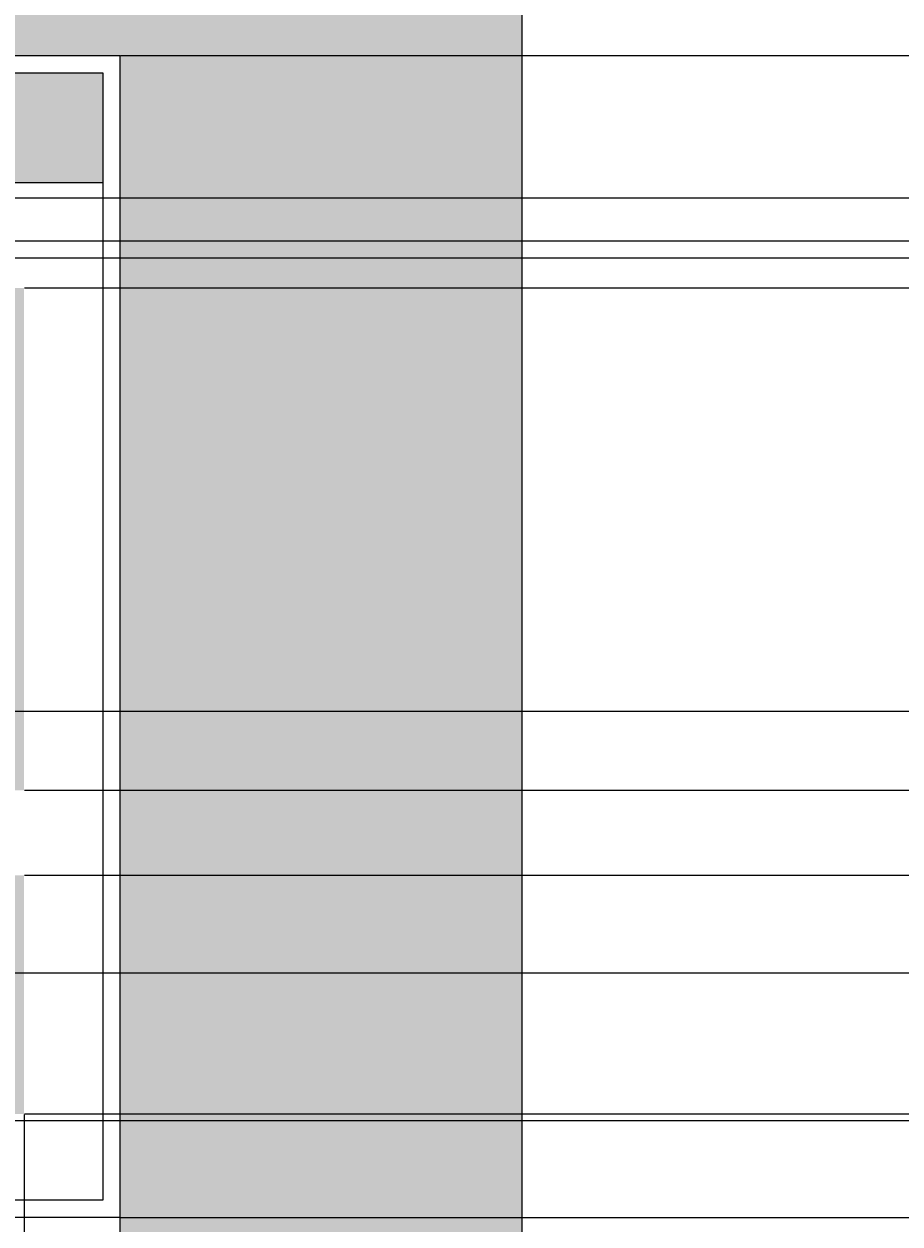
# Model space of a CAD drawing. Units: inches. Extents: x 36 to 594, y 79 to 831.
# Tile 12 of 30: x 390 to 492, y 150 to 290. Entities that reach past the tile are written whole.
import ezdxf

# ---------------------------------------------------------------- set-up
doc = ezdxf.new("R2010")
doc.units = ezdxf.units.IN
doc.header["$MEASUREMENT"] = 0
for name, color, linetype, lineweight in [('A-ANNO-DIMS', 2, 'Continuous', 18), ('A-DOOR', 3, 'Continuous', 18), ('A-ELEV', 7, 'Continuous', 25), ('A-ELEV-PATT', 8, 'Continuous', 13)]:
    doc.layers.add(name, color=color, linetype=linetype, lineweight=lineweight)
doc.styles.get("Standard").update_dxf_attribs({"font": 'arial.ttf'})
doc.dimstyles.get("Standard").update_dxf_attribs({"dimtxt": 0.8125, "dimasz": 0.18, "dimexe": 0.18, "dimexo": 0.0625, "dimgap": 0.09, "dimtad": 0, "dimtih": 1, "dimtoh": 1, "dimdec": 4, "dimzin": 0, "dimdsep": 46, "dimlunit": 4, "dimtxsty": 'Standard', "dimcen": 0.09, "dimadec": 0, "dimazin": 0, "dimtfac": 1, "dimtdec": 4, "dimtofl": 0, "dimtmove": 0, "dimatfit": 3, "dimfxl": 1, "dimtolj": 1, "dimtzin": 0, "dimarcsym": 0})

# ---------------------------------------------------------------- blocks, each defined once
blk = doc.blocks.new('*D30')
at = {"layer": 'A-ANNO-DIMS', "color": 0, "lineweight": -2, "transparency": 16777216}
for p, q in [((401.61, 150.93), (592.85, 150.93)), ((592.67, 150.75), (592.67, 147.08)), ((592.67, 142.39), (592.67, 146.07)), ((401.61, 142.21), (592.85, 142.21))]:
    blk.add_line(p, q, dxfattribs=at)
at = {"layer": 'A-ANNO-DIMS', "color": 0, "transparency": 16777216}
for points in [[(592.64, 150.75), (592.7, 150.75), (592.67, 150.93)], [(592.64, 142.39), (592.7, 142.39), (592.67, 142.21)]]:
    blk.add_solid(points, dxfattribs=at)
at = {"layer": 'Defpoints', "color": 0, "transparency": 16777216}
for p in [(401.55, 150.93), (592.67, 150.93), (401.55, 142.21)]:
    blk.add_point(p, dxfattribs=at)
at = {"layer": 'A-ANNO-DIMS', "color": 0, "transparency": 16777216, "insert": (592.67, 146.57), "char_height": 0.812, "attachment_point": 5}
blk.add_mtext('\\A1;8.722', dxfattribs=at)
blk = doc.blocks.new('*D31')
at = {"layer": 'A-ANNO-DIMS', "color": 0, "lineweight": -2, "transparency": 16777216}
for p, q in [((448.45, 306.21), (592.85, 306.21)), ((592.67, 306.03), (592.67, 229.08)), ((592.67, 151.11), (592.67, 228.07)), ((401.61, 150.93), (592.85, 150.93))]:
    blk.add_line(p, q, dxfattribs=at)
at = {"layer": 'A-ANNO-DIMS', "color": 0, "transparency": 16777216}
for points in [[(592.64, 306.03), (592.7, 306.03), (592.67, 306.21)], [(592.64, 151.11), (592.7, 151.11), (592.67, 150.93)]]:
    blk.add_solid(points, dxfattribs=at)
at = {"layer": 'Defpoints', "color": 0, "transparency": 16777216}
for p in [(448.39, 306.21), (592.67, 306.21), (401.55, 150.93)]:
    blk.add_point(p, dxfattribs=at)
at = {"layer": 'A-ANNO-DIMS', "color": 0, "transparency": 16777216, "insert": (592.67, 228.57), "char_height": 0.812, "attachment_point": 5}
blk.add_mtext('\\A1;155.28', dxfattribs=at)
blk = doc.blocks.new('*D74')
at = {"layer": 'A-ANNO-DIMS', "color": 0, "lineweight": -2, "transparency": 16777216}
for p, q in [((217.09, 179.42), (592.85, 179.42)), ((592.67, 179.24), (592.67, 171.32)), ((592.67, 162.39), (592.67, 170.31)), ((217.09, 162.21), (592.85, 162.21))]:
    blk.add_line(p, q, dxfattribs=at)
at = {"layer": 'A-ANNO-DIMS', "color": 0, "transparency": 16777216}
for points in [[(592.64, 179.24), (592.7, 179.24), (592.67, 179.42)], [(592.64, 162.39), (592.7, 162.39), (592.67, 162.21)]]:
    blk.add_solid(points, dxfattribs=at)
at = {"layer": 'Defpoints', "color": 0, "transparency": 16777216}
for p in [(217.03, 179.42), (592.67, 179.42), (217.03, 162.21)]:
    blk.add_point(p, dxfattribs=at)
at = {"layer": 'A-ANNO-DIMS', "color": 0, "transparency": 16777216, "insert": (592.67, 170.82), "char_height": 0.812, "attachment_point": 5}
blk.add_mtext('\\A1;17.207', dxfattribs=at)
blk = doc.blocks.new('*D75')
at = {"layer": 'A-ANNO-DIMS', "color": 0, "lineweight": -2, "transparency": 16777216}
for p, q in [((215.09, 262.62), (592.85, 262.62)), ((592.67, 262.44), (592.67, 221.53)), ((592.67, 179.6), (592.67, 220.52)), ((217.09, 179.42), (592.85, 179.42))]:
    blk.add_line(p, q, dxfattribs=at)
at = {"layer": 'A-ANNO-DIMS', "color": 0, "transparency": 16777216}
for points in [[(592.64, 262.44), (592.7, 262.44), (592.67, 262.62)], [(592.64, 179.6), (592.7, 179.6), (592.67, 179.42)]]:
    blk.add_solid(points, dxfattribs=at)
at = {"layer": 'Defpoints', "color": 0, "transparency": 16777216}
for p in [(215.03, 262.62), (592.67, 262.62), (217.03, 179.42)]:
    blk.add_point(p, dxfattribs=at)
at = {"layer": 'A-ANNO-DIMS', "color": 0, "transparency": 16777216, "insert": (592.67, 221.02), "char_height": 0.812, "attachment_point": 5}
blk.add_mtext('\\A1;83.2', dxfattribs=at)
blk = doc.blocks.new('*D76')
at = {"layer": 'A-ANNO-DIMS', "color": 0, "lineweight": -2, "transparency": 16777216}
for p, q in [((217.09, 264.62), (592.85, 264.62)), ((592.67, 264.44), (592.67, 264.12)), ((215.09, 262.62), (592.85, 262.62)), ((592.67, 262.8), (592.67, 263.12))]:
    blk.add_line(p, q, dxfattribs=at)
at = {"layer": 'A-ANNO-DIMS', "color": 0, "transparency": 16777216}
for points in [[(592.64, 264.44), (592.7, 264.44), (592.67, 264.62)], [(592.64, 262.8), (592.7, 262.8), (592.67, 262.62)]]:
    blk.add_solid(points, dxfattribs=at)
at = {"layer": 'Defpoints', "color": 0, "transparency": 16777216}
for p in [(217.03, 264.62), (592.67, 264.62), (215.03, 262.62)]:
    blk.add_point(p, dxfattribs=at)
at = {"layer": 'A-ANNO-DIMS', "color": 0, "transparency": 16777216, "insert": (592.67, 263.62), "char_height": 0.812, "attachment_point": 5}
blk.add_mtext('\\A1;2', dxfattribs=at)
blk = doc.blocks.new('*D77')
at = {"layer": 'A-ANNO-DIMS', "color": 0, "lineweight": -2, "transparency": 16777216}
for p, q in [((151.64, 209.88), (592.85, 209.88)), ((592.67, 209.7), (592.67, 186.55)), ((592.67, 162.39), (592.67, 185.54)), ((156.47, 162.21), (592.85, 162.21))]:
    blk.add_line(p, q, dxfattribs=at)
at = {"layer": 'A-ANNO-DIMS', "color": 0, "transparency": 16777216}
for points in [[(592.64, 209.7), (592.7, 209.7), (592.67, 209.88)], [(592.64, 162.39), (592.7, 162.39), (592.67, 162.21)]]:
    blk.add_solid(points, dxfattribs=at)
at = {"layer": 'Defpoints', "color": 0, "transparency": 16777216}
for p in [(151.58, 209.88), (156.41, 162.21), (592.67, 162.21)]:
    blk.add_point(p, dxfattribs=at)
at = {"layer": 'A-ANNO-DIMS', "color": 0, "transparency": 16777216, "insert": (592.67, 186.05), "char_height": 0.812, "attachment_point": 5}
blk.add_mtext('\\A1;47.67', dxfattribs=at)
blk = doc.blocks.new('*D82')
at = {"layer": 'A-ANNO-DIMS', "color": 0, "lineweight": -2, "transparency": 16777216}
for p, q in [((335.35, 162.93), (335.35, 79.53)), ((390.39, 162.93), (390.39, 79.53)), ((335.53, 79.71), (361.41, 79.71)), ((390.21, 79.71), (364.33, 79.71))]:
    blk.add_line(p, q, dxfattribs=at)
at = {"layer": 'A-ANNO-DIMS', "color": 0, "transparency": 16777216}
for points in [[(335.53, 79.74), (335.53, 79.68), (335.35, 79.71)], [(390.21, 79.74), (390.21, 79.68), (390.39, 79.71)]]:
    blk.add_solid(points, dxfattribs=at)
at = {"layer": 'Defpoints', "color": 0, "transparency": 16777216}
for p in [(335.35, 162.99), (390.39, 162.99), (390.39, 79.71)]:
    blk.add_point(p, dxfattribs=at)
at = {"layer": 'A-ANNO-DIMS', "color": 0, "transparency": 16777216, "insert": (362.87, 79.71), "char_height": 0.812, "attachment_point": 5}
blk.add_mtext('\\A1;55.04', dxfattribs=at)
blk = doc.blocks.new('*D83')
at = {"layer": 'A-ANNO-DIMS', "color": 0, "lineweight": -2, "transparency": 16777216}
for p, q in [((390.39, 162.93), (390.39, 79.53)), ((401.55, 150.87), (401.55, 79.53)), ((390.57, 79.71), (394.23, 79.71)), ((401.37, 79.71), (397.71, 79.71))]:
    blk.add_line(p, q, dxfattribs=at)
at = {"layer": 'A-ANNO-DIMS', "color": 0, "transparency": 16777216}
for points in [[(390.57, 79.74), (390.57, 79.68), (390.39, 79.71)], [(401.37, 79.74), (401.37, 79.68), (401.55, 79.71)]]:
    blk.add_solid(points, dxfattribs=at)
at = {"layer": 'Defpoints', "color": 0, "transparency": 16777216}
for p in [(390.39, 162.99), (401.55, 150.93), (401.55, 79.71)]:
    blk.add_point(p, dxfattribs=at)
at = {"layer": 'A-ANNO-DIMS', "color": 0, "transparency": 16777216, "insert": (395.97, 79.71), "char_height": 0.812, "attachment_point": 5}
blk.add_mtext('\\A1;11.163', dxfattribs=at)
blk = doc.blocks.new('*D84')
at = {"layer": 'A-ANNO-DIMS', "color": 0, "lineweight": -2, "transparency": 16777216}
for p, q in [((390.45, 162.99), (592.85, 162.99)), ((592.67, 162.81), (592.67, 157.47)), ((592.67, 151.11), (592.67, 156.46)), ((401.61, 150.93), (592.85, 150.93))]:
    blk.add_line(p, q, dxfattribs=at)
at = {"layer": 'A-ANNO-DIMS', "color": 0, "transparency": 16777216}
for points in [[(592.64, 162.81), (592.7, 162.81), (592.67, 162.99)], [(592.64, 151.11), (592.7, 151.11), (592.67, 150.93)]]:
    blk.add_solid(points, dxfattribs=at)
at = {"layer": 'Defpoints', "color": 0, "transparency": 16777216}
for p in [(390.39, 162.99), (592.67, 162.99), (401.55, 150.93)]:
    blk.add_point(p, dxfattribs=at)
at = {"layer": 'A-ANNO-DIMS', "color": 0, "transparency": 16777216, "insert": (592.67, 156.96), "char_height": 0.812, "attachment_point": 5}
blk.add_mtext('\\A1;12.053', dxfattribs=at)
blk = doc.blocks.new('*D85')
at = {"layer": 'A-ANNO-DIMS', "color": 0, "lineweight": -2, "transparency": 16777216}
for p, q in [((390.45, 190.77), (592.85, 190.77)), ((592.67, 190.59), (592.67, 177.38)), ((592.67, 163.17), (592.67, 176.37)), ((390.45, 162.99), (592.85, 162.99))]:
    blk.add_line(p, q, dxfattribs=at)
at = {"layer": 'A-ANNO-DIMS', "color": 0, "transparency": 16777216}
for points in [[(592.64, 190.59), (592.7, 190.59), (592.67, 190.77)], [(592.64, 163.17), (592.7, 163.17), (592.67, 162.99)]]:
    blk.add_solid(points, dxfattribs=at)
at = {"layer": 'Defpoints', "color": 0, "transparency": 16777216}
for p in [(390.39, 190.77), (592.67, 190.77), (390.39, 162.99)]:
    blk.add_point(p, dxfattribs=at)
at = {"layer": 'A-ANNO-DIMS', "color": 0, "transparency": 16777216, "insert": (592.67, 176.88), "char_height": 0.812, "attachment_point": 5}
blk.add_mtext('\\A1;27.78', dxfattribs=at)
blk = doc.blocks.new('*D86')
at = {"layer": 'A-ANNO-DIMS', "color": 0, "lineweight": -2, "transparency": 16777216}
for p, q in [((390.45, 200.66), (592.85, 200.66)), ((592.67, 200.48), (592.67, 196.22)), ((592.67, 190.95), (592.67, 195.21)), ((390.45, 190.77), (592.85, 190.77))]:
    blk.add_line(p, q, dxfattribs=at)
at = {"layer": 'A-ANNO-DIMS', "color": 0, "transparency": 16777216}
for points in [[(592.64, 200.48), (592.7, 200.48), (592.67, 200.66)], [(592.64, 190.95), (592.7, 190.95), (592.67, 190.77)]]:
    blk.add_solid(points, dxfattribs=at)
at = {"layer": 'Defpoints', "color": 0, "transparency": 16777216}
for p in [(390.39, 200.66), (592.67, 200.66), (390.39, 190.77)]:
    blk.add_point(p, dxfattribs=at)
at = {"layer": 'A-ANNO-DIMS', "color": 0, "transparency": 16777216, "insert": (592.67, 195.72), "char_height": 0.812, "attachment_point": 5}
blk.add_mtext('\\A1;9.895', dxfattribs=at)
blk = doc.blocks.new('*D87')
at = {"layer": 'A-ANNO-DIMS', "color": 0, "lineweight": -2, "transparency": 16777216}
for p, q in [((390.45, 259.12), (592.85, 259.12)), ((592.67, 258.94), (592.67, 230.4)), ((592.67, 200.84), (592.67, 229.39)), ((390.45, 200.66), (592.85, 200.66))]:
    blk.add_line(p, q, dxfattribs=at)
at = {"layer": 'A-ANNO-DIMS', "color": 0, "transparency": 16777216}
for points in [[(592.64, 258.94), (592.7, 258.94), (592.67, 259.12)], [(592.64, 200.84), (592.7, 200.84), (592.67, 200.66)]]:
    blk.add_solid(points, dxfattribs=at)
at = {"layer": 'Defpoints', "color": 0, "transparency": 16777216}
for p in [(390.39, 259.12), (592.67, 259.12), (390.39, 200.66)]:
    blk.add_point(p, dxfattribs=at)
at = {"layer": 'A-ANNO-DIMS', "color": 0, "transparency": 16777216, "insert": (592.67, 229.89), "char_height": 0.812, "attachment_point": 5}
blk.add_mtext('\\A1;58.46', dxfattribs=at)
blk = doc.blocks.new('*D88')
at = {"layer": 'A-ANNO-DIMS', "color": 0, "lineweight": -2, "transparency": 16777216}
for p, q in [((399.61, 269.61), (592.85, 269.61)), ((592.67, 269.43), (592.67, 264.87)), ((592.67, 259.3), (592.67, 263.86)), ((390.45, 259.12), (592.85, 259.12))]:
    blk.add_line(p, q, dxfattribs=at)
at = {"layer": 'A-ANNO-DIMS', "color": 0, "transparency": 16777216}
for points in [[(592.64, 269.43), (592.7, 269.43), (592.67, 269.61)], [(592.64, 259.3), (592.7, 259.3), (592.67, 259.12)]]:
    blk.add_solid(points, dxfattribs=at)
at = {"layer": 'Defpoints', "color": 0, "transparency": 16777216}
for p in [(399.55, 269.61), (592.67, 269.61), (390.39, 259.12)]:
    blk.add_point(p, dxfattribs=at)
at = {"layer": 'A-ANNO-DIMS', "color": 0, "transparency": 16777216, "insert": (592.67, 264.37), "char_height": 0.812, "attachment_point": 5}
blk.add_mtext('\\A1;10.484', dxfattribs=at)
blk = doc.blocks.new('*D89')
at = {"layer": 'A-ANNO-DIMS', "color": 0, "lineweight": -2, "transparency": 16777216}
for p, q in [((401.61, 286.18), (592.85, 286.18)), ((592.67, 286), (592.67, 278.4)), ((592.67, 269.79), (592.67, 277.39)), ((399.61, 269.61), (592.85, 269.61))]:
    blk.add_line(p, q, dxfattribs=at)
at = {"layer": 'A-ANNO-DIMS', "color": 0, "transparency": 16777216}
for points in [[(592.64, 286), (592.7, 286), (592.67, 286.18)], [(592.64, 269.79), (592.7, 269.79), (592.67, 269.61)]]:
    blk.add_solid(points, dxfattribs=at)
at = {"layer": 'Defpoints', "color": 0, "transparency": 16777216}
for p in [(401.55, 286.18), (592.67, 286.18), (399.55, 269.61)]:
    blk.add_point(p, dxfattribs=at)
at = {"layer": 'A-ANNO-DIMS', "color": 0, "transparency": 16777216, "insert": (592.67, 277.89), "char_height": 0.812, "attachment_point": 5}
blk.add_mtext('\\A1;16.572', dxfattribs=at)

msp = doc.modelspace()

# ---------------------------------------------------------------- hatches: boundary and pattern name
at = {"layer": 'A-ELEV-PATT'}
h = msp.add_hatch(color=256, dxfattribs=at)
h.dxf.hatch_style = 1
h.paths.add_polyline_path([(398.0873, 796.0465), (269.3592, 796.0465), (269.3592, 770.1455), (397.8159, 770.1455)])
h.paths.add_polyline_path([(397.7518, 764.0341), (269.3592, 764.0341), (269.3592, 630.0394), (341.8367, 630.0394), (341.8367, 720.595), (335.0881, 728.3699), (329.982, 735.3373), (345.3661, 727.7743), (397.1052, 702.3389)])
h.paths.add_polyline_path([(341.8367, 594.2124), (201.4189, 594.2124), (201.4189, 475.4136), (232.8216, 475.4136), (232.8216, 524.6037), (341.8367, 524.6037)])
h.paths.add_polyline_path([(177.525, 594.2124), (118.7598, 594.2124), (118.7598, 450.2124), (177.525, 450.2124)])
h.paths.add_polyline_path([(424.4958, 594.2124), (365.7306, 594.2124), (365.7306, 450.2124), (424.4958, 450.2124)])
h.paths.add_polyline_path([(241.3553, 404.2737), (355.8569, 404.2737), (355.8569, 355.0836), (424.5492, 355.0836), (424.5492, 425.7333), (118.7598, 426.2844), (118.7598, 355.0836), (241.3553, 355.0836)])
h.paths.add_polyline_path([(448.3898, 306.2124), (217.0273, 306.2124), (217.0273, 142.2124), (254.0293, 142.2124), (254.0293, 150.9347), (254.0293, 286.1802), (401.5491, 286.1802), (401.5491, 150.9347), (401.5491, 142.2124), (448.3898, 142.2124)])
h.paths.add_polyline_path([(448.3898, 142.2124), (401.5491, 142.2124), (217.0273, 142.2124), (217.0273, 114.2124), (448.3898, 114.2124)])
h.paths.add_polyline_path([(217.0273, 306.2124), (174.7353, 306.2124), (94.8658, 306.2124), (94.8658, 162.2124), (103.3368, 162.2124), (103.3368, 264.6224), (103.3368, 286.1802), (217.0273, 286.1802)])
h = msp.add_hatch(color=256, dxfattribs=at)
h.dxf.hatch_style = 1
h.set_gradient(color1=(0, 255, 255), color2=(16, 86, 137))
h.paths.add_polyline_path([(341.8367, 524.6037), (260.5056, 524.6037), (260.5056, 513.1224), (341.8367, 513.1224)])
h.paths.add_polyline_path([(341.8367, 511.1224), (260.5056, 511.1224), (260.5056, 475.4136), (341.8367, 475.4136)])
h.paths.add_polyline_path([(258.5056, 524.6037), (232.8216, 524.6037), (232.8216, 513.1224), (258.5056, 513.1224)])
h.paths.add_polyline_path([(355.8569, 404.2737), (269.0393, 404.2737), (269.0393, 392.7924), (355.8569, 392.7924)])
h.paths.add_polyline_path([(267.0393, 404.2737), (241.3553, 404.2737), (241.3553, 392.7924), (267.0393, 392.7924)])
h.paths.add_polyline_path([(355.8569, 390.7924), (269.0393, 390.7924), (269.0393, 355.0836), (355.8569, 355.0836)])
h.paths.add_polyline_path([(399.5491, 284.1802), (256.0293, 284.1802), (256.0293, 271.378), (399.5491, 271.378)])
h.paths.add_polyline_path([(317.3533, 259.1243), (262.3169, 259.1243), (262.3169, 200.6645), (317.3533, 200.6645)])
h.paths.add_polyline_path([(390.386, 259.1243), (335.3496, 259.1243), (335.3496, 200.6645), (390.386, 200.6645)])
h.paths.add_polyline_path([(390.386, 190.7697), (335.3496, 190.7697), (335.3496, 162.9881), (390.386, 162.9881)])
h.paths.add_polyline_path([(317.3533, 190.7697), (262.3169, 190.7697), (262.3169, 162.9881), (317.3533, 162.9881)])
h.paths.add_polyline_path([(215.0273, 262.6224), (158.4069, 262.6224), (158.4069, 181.4195), (215.0273, 181.4195)])
h.paths.add_polyline_path([(215.0273, 284.1802), (105.3368, 284.1802), (105.3368, 266.6224), (215.0273, 266.6224)])

# ---------------------------------------------------------------- linework, layer by layer
at = {"layer": 'A-DOOR'}
msp.add_line((256.0293, 271.378), (399.5491, 271.378), dxfattribs=at)
for points in [[(254.0293, 286.1802), (401.5491, 286.1802), (401.5491, 150.9347), (254.0293, 150.9347)], [(256.0293, 284.1802), (399.5491, 284.1802), (399.5491, 152.9347), (256.0293, 152.9347)], [(327.7892, 269.6084), (399.5491, 269.6084), (399.5491, 152.9347), (327.7892, 152.9347)]]:
    msp.add_lwpolyline(points, close=True, dxfattribs=at)
at = {"layer": 'A-ELEV'}
for p, q in [((448.3898, 142.2124), (448.3898, 367.5118)), ((401.5491, 150.9347), (401.5491, 142.2124))]:
    msp.add_line(p, q, dxfattribs=at)

# ---------------------------------------------------------------- dimensions: what is measured, and where the dimension line sits
at = {"layer": 'A-ANNO-DIMS'}
for base, p1, p2, override, picture, middle in [((592.6689, 306.2124), (401.5491, 150.9347), (448.3898, 306.2124), {"dimdec": 2, "dimlfac": 1, "dimrnd": 0, "dimzin": 0, "dimdsep": 46, "dimlunit": 2}, '*D31', (592.6689, 228.5735)), ((592.6689, 286.1802), (399.5491, 269.6084), (401.5491, 286.1802), {"dimdec": 3, "dimlfac": 1, "dimrnd": 0, "dimzin": 0, "dimdsep": 46, "dimlunit": 2}, '*D89', (592.6689, 277.8943)), ((592.6689, 269.6084), (390.386, 259.1243), (399.5491, 269.6084), {"dimdec": 3, "dimlfac": 1, "dimrnd": 0, "dimzin": 0, "dimdsep": 46, "dimlunit": 2}, '*D88', (592.6689, 264.3664)), ((592.6689, 264.6224), (215.0273, 262.6224), (217.0273, 264.6224), {"dimdec": 0, "dimlfac": 1, "dimrnd": 0, "dimzin": 0, "dimdsep": 46, "dimlunit": 2}, '*D76', (592.6689, 263.6224)), ((592.6689, 262.6224), (217.0273, 179.4195), (215.0273, 262.6224), {"dimdec": 1, "dimlfac": 1, "dimrnd": 0, "dimzin": 0, "dimdsep": 46, "dimlunit": 2}, '*D75', (592.6689, 221.021)), ((592.6689, 259.1243), (390.386, 200.6645), (390.386, 259.1243), {"dimdec": 2, "dimlfac": 1, "dimrnd": 0, "dimzin": 0, "dimdsep": 46, "dimlunit": 2}, '*D87', (592.6689, 229.8944)), ((592.6689, 162.2124), (151.5799, 209.8823), (156.4069, 162.2124), {"dimdec": 2, "dimlfac": 1, "dimrnd": 0, "dimzin": 0, "dimdsep": 46, "dimlunit": 2}, '*D77', (592.6689, 186.0473)), ((592.6689, 200.6645), (390.386, 190.7697), (390.386, 200.6645), {"dimdec": 3, "dimlfac": 1, "dimrnd": 0, "dimzin": 0, "dimdsep": 46, "dimlunit": 2}, '*D86', (592.6689, 195.7171)), ((592.6689, 190.7697), (390.386, 162.9881), (390.386, 190.7697), {"dimdec": 2, "dimlfac": 1, "dimrnd": 0, "dimzin": 0, "dimdsep": 46, "dimlunit": 2}, '*D85', (592.6689, 176.8789)), ((592.6689, 179.4195), (217.0273, 162.2124), (217.0273, 179.4195), {"dimdec": 3, "dimlfac": 1, "dimrnd": 0, "dimzin": 0, "dimdsep": 46, "dimlunit": 2}, '*D74', (592.6689, 170.8159)), ((592.6689, 162.9881), (401.5491, 150.9347), (390.386, 162.9881), {"dimdec": 3, "dimlfac": 1, "dimrnd": 0, "dimzin": 0, "dimdsep": 46, "dimlunit": 2}, '*D84', (592.6689, 156.9614)), ((592.6689, 150.9347), (401.5491, 142.2124), (401.5491, 150.9347), {"dimdec": 3, "dimlfac": 1, "dimrnd": 0, "dimzin": 0, "dimdsep": 46, "dimlunit": 2}, '*D30', (592.6689, 146.5735))]:
    dim = msp.add_linear_dim(base=base, p1=p1, p2=p2, angle=90, dimstyle='Standard', override=override, dxfattribs=at)
    dim.commit()
    dim.dimension.update_dxf_attribs({"geometry": picture, "text_midpoint": middle})
for base, p1, p2, override, picture, middle in [((390.386, 79.7124), (335.3496, 162.9881), (390.386, 162.9881), {"dimdec": 2, "dimlfac": 1, "dimrnd": 0, "dimzin": 0, "dimdsep": 46, "dimlunit": 2}, '*D82', (362.8678, 79.7124)), ((401.5491, 79.7124), (390.386, 162.9881), (401.5491, 150.9347), {"dimdec": 3, "dimlfac": 1, "dimrnd": 0, "dimzin": 0, "dimdsep": 46, "dimlunit": 2}, '*D83', (395.9676, 79.7124))]:
    dim = msp.add_linear_dim(base=base, p1=p1, p2=p2, dimstyle='Standard', override=override, dxfattribs=at)
    dim.commit()
    dim.dimension.update_dxf_attribs({"geometry": picture, "text_midpoint": middle})

doc.saveas('drawing.dxf')
